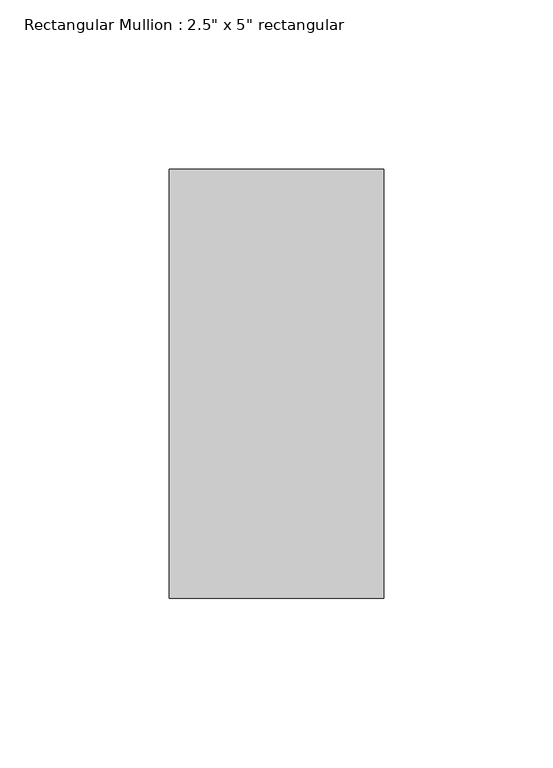
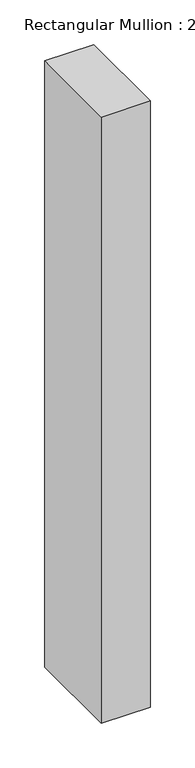
"""IFC4 building model written with IfcOpenShell, lengths in millimetres: member geometry."""

from ifc_helpers import new_model, si_unit, frame, origin, place, context, project, spatial, polyline, outline, extrude, source, transform, mapped, element, save


def member_9b02ea12(model_context):
    return source(origin(), model_context, "Body", "SweptSolid", [
        extrude(outline(polyline([(31.75, 63.5), (31.75, -63.5), (-31.75, -63.5), (-31.75, 63.5), (31.75, 63.5)])), frame((0.0, 0.0, -830.6744987), z_axis=(0.0, 0.0, 1.0), x_axis=(1.0, 0.0, 0.0)), (0.0, 0.0, 1.0), 830.6744987),
    ])


if __name__ == "__main__":
    model = new_model("IFC4")
    model_context = context("Model", 3, world=origin())
    ifc_project = project(units=[si_unit("LENGTHUNIT", "METRE", prefix="MILLI")], contexts=[model_context])
    site = spatial("IfcSite", under=ifc_project)
    building = spatial("IfcBuilding", under=site)
    placement = place(None, origin())
    member_shape = member_9b02ea12(model_context)
    element("IfcMember", 1, ObjectType="Rectangular Mullion : 2.5\" x 5\" rectangular", at=placement, inside=building, context=model_context, shape_type="MappedRepresentation", body=[
        mapped(member_shape, transform((0.0, 0.0, 0.0), x_axis=(1.0, 0.0, 0.0), y_axis=(0.0, 1.0, 0.0), z_axis=(0.0, 0.0, 1.0))),
    ])
    save(model, "model.ifc")

# Revit data of these elements
# Type "Rectangular Mullion : 2.5\" x 5\" rectangular"
#   built-in parameter 1007304 = 0.416667 (stored number, unit not read)
#   built-in parameter 1007301 = 0.104167 (stored number, unit not read)
#   built-in parameter 1007300 = 0.104167 (stored number, unit not read)
# Element 1 (IfcMember, "Rectangular Mullion : 2.5\" x 5\" rectangular")
#   Materials on its faces: "Aluminum"
# Materials
#   "Aluminum": class "Metal", colour RGB 247 247 247, transparency 0, Description = "Aluminum 6061", Cost = 0
